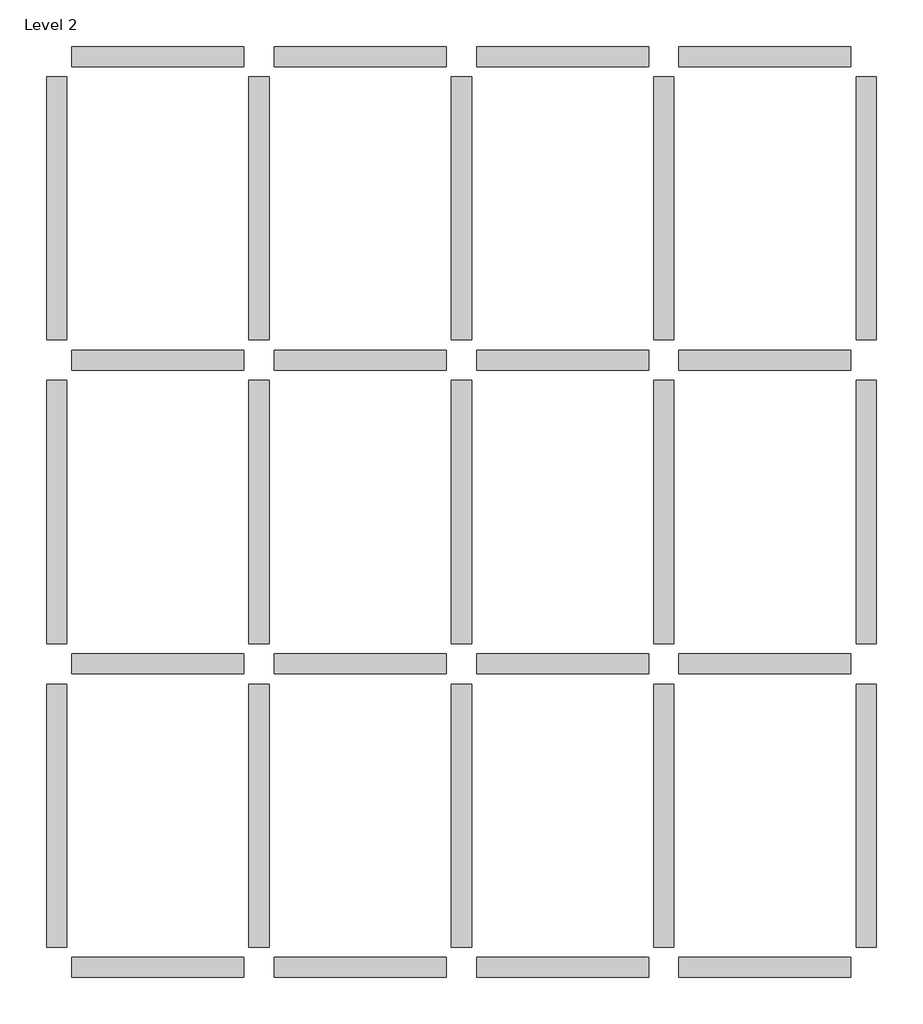
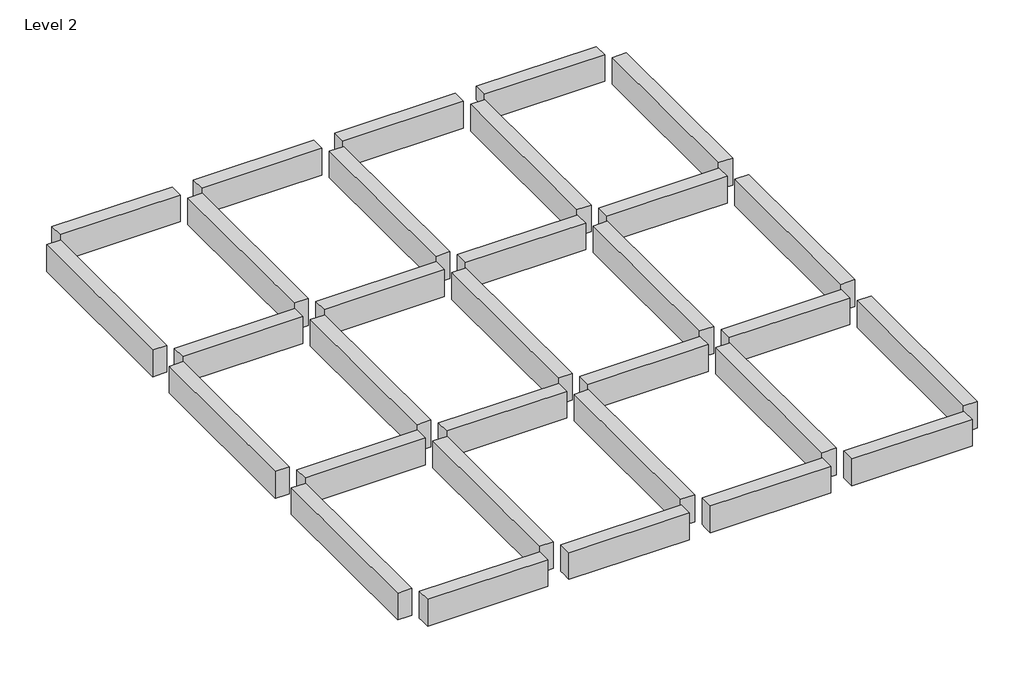
# One storey: 31 beams.
"""IFC4 building model written with IfcOpenShell, lengths in millimetres."""

from ifc_helpers import new_model, si_unit, frame, origin, place, context, project, spatial, polyline, outline, extrude, faceted_brep, element, save

model = new_model("IFC4")

# Units and contexts
model_context = context("Model", 3, world=origin())
ifc_project = project(units=[si_unit("LENGTHUNIT", "METRE", prefix="MILLI")], contexts=[model_context])

# Site, building, storey
site = spatial("IfcSite", under=ifc_project)
building = spatial("IfcBuilding", under=site)
storey = spatial("IfcBuildingStorey", under=building, Name="Level 2", Elevation=3048.0)

# Beams
placement = place(None, origin())
element("IfcBeam", 1, ObjectType="Concrete-Rectangular Beam : 12 x 24", at=placement, inside=storey, context=model_context, shape_type="Brep", body=[
    faceted_brep([(-21467.3183349, 4163.0075069, 3048.0), (-21772.1183349, 4163.0075069, 3048.0), (-21772.1183349, 200.6075069, 3048.0), (-21467.3183349, 200.6075069, 3048.0), (-21467.3183349, 4163.0075069, 2438.4), (-21467.3183349, 200.6075069, 2438.4), (-21772.1183349, 4163.0075069, 2438.4), (-21568.9183349, 4163.0075069, 2438.4), (-21568.9183349, 200.6075069, 2438.4), (-21772.1183349, 200.6075069, 2438.4)], [[[0, 1, 2, 3]], [[4, 0, 3, 5]], [[6, 7, 4, 5, 8, 9]], [[1, 6, 9, 2]], [[1, 0, 4, 7, 6]], [[3, 2, 9, 8, 5]]]),
])
element("IfcBeam", 2, ObjectType="Concrete-Rectangular Beam : 12 x 24", at=placement, inside=storey, context=model_context, shape_type="Brep", body=[
    faceted_brep([(-21467.3183349, 8735.0075069, 3048.0), (-21772.1183349, 8735.0075069, 3048.0), (-21772.1183349, 4772.6075069, 3048.0), (-21467.3183349, 4772.6075069, 3048.0), (-21467.3183349, 8735.0075069, 2438.4), (-21467.3183349, 4772.6075069, 2438.4), (-21772.1183349, 8735.0075069, 2438.4), (-21568.9183349, 8735.0075069, 2438.4), (-21568.9183349, 4772.6075069, 2438.4), (-21772.1183349, 4772.6075069, 2438.4)], [[[0, 1, 2, 3]], [[4, 0, 3, 5]], [[6, 7, 4, 5, 8, 9]], [[1, 6, 9, 2]], [[1, 0, 4, 7, 6]], [[3, 2, 9, 8, 5]]]),
])
element("IfcBeam", 3, ObjectType="Concrete-Rectangular Beam : 12 x 24", at=placement, inside=storey, context=model_context, shape_type="Brep", body=[
    faceted_brep([(-21467.3183349, 13307.0075069, 3048.0), (-21772.1183349, 13307.0075069, 3048.0), (-21772.1183349, 9344.6075069, 3048.0), (-21467.3183349, 9344.6075069, 3048.0), (-21467.3183349, 13307.0075069, 2438.4), (-21467.3183349, 9344.6075069, 2438.4), (-21772.1183349, 13307.0075069, 2438.4), (-21568.9183349, 13307.0075069, 2438.4), (-21568.9183349, 9344.6075069, 2438.4), (-21772.1183349, 9344.6075069, 2438.4)], [[[0, 1, 2, 3]], [[4, 0, 3, 5]], [[6, 7, 4, 5, 8, 9]], [[1, 6, 9, 2]], [[1, 0, 4, 7, 6]], [[3, 2, 9, 8, 5]]]),
])
element("IfcBeam", 4, ObjectType="Concrete-Rectangular Beam : 12 x 24", at=placement, inside=storey, context=model_context, shape_type="SweptSolid", body=[
    extrude(outline(polyline([(-18724.1183349, 4163.0075069), (-18419.3183349, 4163.0075069), (-18419.3183349, 200.6075069), (-18724.1183349, 200.6075069), (-18724.1183349, 4163.0075069)])), frame((0.0, 0.0, 2438.4), z_axis=(0.0, 0.0, 1.0), x_axis=(1.0, 0.0, 0.0)), (0.0, 0.0, 1.0), 609.6),
])
element("IfcBeam", 5, ObjectType="Concrete-Rectangular Beam : 12 x 24", at=placement, inside=storey, context=model_context, shape_type="SweptSolid", body=[
    extrude(outline(polyline([(-18724.1183349, 8735.0075069), (-18419.3183349, 8735.0075069), (-18419.3183349, 4772.6075069), (-18724.1183349, 4772.6075069), (-18724.1183349, 8735.0075069)])), frame((0.0, 0.0, 2438.4), z_axis=(0.0, 0.0, 1.0), x_axis=(1.0, 0.0, 0.0)), (0.0, 0.0, 1.0), 609.6),
])
element("IfcBeam", 6, ObjectType="Concrete-Rectangular Beam : 12 x 24", at=placement, inside=storey, context=model_context, shape_type="SweptSolid", body=[
    extrude(outline(polyline([(-18724.1183349, 13307.0075069), (-18419.3183349, 13307.0075069), (-18419.3183349, 9344.6075069), (-18724.1183349, 9344.6075069), (-18724.1183349, 13307.0075069)])), frame((0.0, 0.0, 2438.4), z_axis=(0.0, 0.0, 1.0), x_axis=(1.0, 0.0, 0.0)), (0.0, 0.0, 1.0), 609.6),
])
element("IfcBeam", 7, ObjectType="Concrete-Rectangular Beam : 12 x 24", at=placement, inside=storey, context=model_context, shape_type="SweptSolid", body=[
    extrude(outline(polyline([(-15676.1183349, 4163.0075069), (-15371.3183349, 4163.0075069), (-15371.3183349, 200.6075069), (-15676.1183349, 200.6075069), (-15676.1183349, 4163.0075069)])), frame((0.0, 0.0, 2438.4), z_axis=(0.0, 0.0, 1.0), x_axis=(1.0, 0.0, 0.0)), (0.0, 0.0, 1.0), 609.6),
])
element("IfcBeam", 8, ObjectType="Concrete-Rectangular Beam : 12 x 24", at=placement, inside=storey, context=model_context, shape_type="SweptSolid", body=[
    extrude(outline(polyline([(-15676.1183349, 8735.0075069), (-15371.3183349, 8735.0075069), (-15371.3183349, 4772.6075069), (-15676.1183349, 4772.6075069), (-15676.1183349, 8735.0075069)])), frame((0.0, 0.0, 2438.4), z_axis=(0.0, 0.0, 1.0), x_axis=(1.0, 0.0, 0.0)), (0.0, 0.0, 1.0), 609.6),
])
element("IfcBeam", 9, ObjectType="Concrete-Rectangular Beam : 12 x 24", at=placement, inside=storey, context=model_context, shape_type="SweptSolid", body=[
    extrude(outline(polyline([(-15676.1183349, 13307.0075069), (-15371.3183349, 13307.0075069), (-15371.3183349, 9344.6075069), (-15676.1183349, 9344.6075069), (-15676.1183349, 13307.0075069)])), frame((0.0, 0.0, 2438.4), z_axis=(0.0, 0.0, 1.0), x_axis=(1.0, 0.0, 0.0)), (0.0, 0.0, 1.0), 609.6),
])
element("IfcBeam", 10, ObjectType="Concrete-Rectangular Beam : 12 x 24", at=placement, inside=storey, context=model_context, shape_type="SweptSolid", body=[
    extrude(outline(polyline([(-12628.1183349, 4163.0075069), (-12323.3183349, 4163.0075069), (-12323.3183349, 200.6075069), (-12628.1183349, 200.6075069), (-12628.1183349, 4163.0075069)])), frame((0.0, 0.0, 2438.4), z_axis=(0.0, 0.0, 1.0), x_axis=(1.0, 0.0, 0.0)), (0.0, 0.0, 1.0), 609.6),
])
element("IfcBeam", 11, ObjectType="Concrete-Rectangular Beam : 12 x 24", at=placement, inside=storey, context=model_context, shape_type="SweptSolid", body=[
    extrude(outline(polyline([(-12628.1183349, 8735.0075069), (-12323.3183349, 8735.0075069), (-12323.3183349, 4772.6075069), (-12628.1183349, 4772.6075069), (-12628.1183349, 8735.0075069)])), frame((0.0, 0.0, 2438.4), z_axis=(0.0, 0.0, 1.0), x_axis=(1.0, 0.0, 0.0)), (0.0, 0.0, 1.0), 609.6),
])
element("IfcBeam", 12, ObjectType="Concrete-Rectangular Beam : 12 x 24", at=placement, inside=storey, context=model_context, shape_type="SweptSolid", body=[
    extrude(outline(polyline([(-12628.1183349, 13307.0075069), (-12323.3183349, 13307.0075069), (-12323.3183349, 9344.6075069), (-12628.1183349, 9344.6075069), (-12628.1183349, 13307.0075069)])), frame((0.0, 0.0, 2438.4), z_axis=(0.0, 0.0, 1.0), x_axis=(1.0, 0.0, 0.0)), (0.0, 0.0, 1.0), 609.6),
])
element("IfcBeam", 13, ObjectType="Concrete-Rectangular Beam : 12 x 24", at=placement, inside=storey, context=model_context, shape_type="Brep", body=[
    faceted_brep([(-9275.3183349, 4163.0075069, 3048.0), (-9580.1183349, 4163.0075069, 3048.0), (-9580.1183349, 200.6075069, 3048.0), (-9275.3183349, 200.6075069, 3048.0), (-9275.3183349, 4163.0075069, 2438.4), (-9275.3183349, 200.6075069, 2438.4), (-9580.1183349, 4163.0075069, 2438.4), (-9478.5183349, 4163.0075069, 2438.4), (-9478.5183349, 200.6075069, 2438.4), (-9580.1183349, 200.6075069, 2438.4)], [[[0, 1, 2, 3]], [[4, 0, 3, 5]], [[6, 7, 4, 5, 8, 9]], [[1, 6, 9, 2]], [[1, 0, 4, 7, 6]], [[3, 2, 9, 8, 5]]]),
])
element("IfcBeam", 14, ObjectType="Concrete-Rectangular Beam : 12 x 24", at=placement, inside=storey, context=model_context, shape_type="Brep", body=[
    faceted_brep([(-9275.3183349, 8735.0075069, 3048.0), (-9580.1183349, 8735.0075069, 3048.0), (-9580.1183349, 4772.6075069, 3048.0), (-9275.3183349, 4772.6075069, 3048.0), (-9275.3183349, 8735.0075069, 2438.4), (-9275.3183349, 4772.6075069, 2438.4), (-9580.1183349, 8735.0075069, 2438.4), (-9478.5183349, 8735.0075069, 2438.4), (-9478.5183349, 4772.6075069, 2438.4), (-9580.1183349, 4772.6075069, 2438.4)], [[[0, 1, 2, 3]], [[4, 0, 3, 5]], [[6, 7, 4, 5, 8, 9]], [[1, 6, 9, 2]], [[1, 0, 4, 7, 6]], [[3, 2, 9, 8, 5]]]),
])
element("IfcBeam", 15, ObjectType="Concrete-Rectangular Beam : 12 x 24", at=placement, inside=storey, context=model_context, shape_type="Brep", body=[
    faceted_brep([(-9275.3183349, 13307.0075069, 3048.0), (-9580.1183349, 13307.0075069, 3048.0), (-9580.1183349, 9344.6075069, 3048.0), (-9275.3183349, 9344.6075069, 3048.0), (-9275.3183349, 13307.0075069, 2438.4), (-9275.3183349, 9344.6075069, 2438.4), (-9580.1183349, 13307.0075069, 2438.4), (-9478.5183349, 13307.0075069, 2438.4), (-9478.5183349, 9344.6075069, 2438.4), (-9580.1183349, 9344.6075069, 2438.4)], [[[0, 1, 2, 3]], [[4, 0, 3, 5]], [[6, 7, 4, 5, 8, 9]], [[1, 6, 9, 2]], [[1, 0, 4, 7, 6]], [[3, 2, 9, 8, 5]]]),
])
element("IfcBeam", 16, ObjectType="Concrete-Rectangular Beam : 12 x 24", at=placement, inside=storey, context=model_context, shape_type="Brep", body=[
    faceted_brep([(-21391.1183349, 13764.2075069, 3048.0), (-21391.1183349, 13459.4075069, 3048.0), (-18800.3183349, 13459.4075069, 3048.0), (-18800.3183349, 13764.2075069, 3048.0), (-21391.1183349, 13459.4075069, 2438.4), (-18800.3183349, 13459.4075069, 2438.4), (-21391.1183349, 13561.0075069, 2438.4), (-21391.1183349, 13764.2075069, 2438.4), (-18800.3183349, 13764.2075069, 2438.4), (-18800.3183349, 13561.0075069, 2438.4)], [[[0, 1, 2, 3]], [[1, 4, 5, 2]], [[4, 6, 7, 8, 9, 5]], [[7, 0, 3, 8]], [[1, 0, 7, 6, 4]], [[3, 2, 5, 9, 8]]]),
])
element("IfcBeam", 17, ObjectType="Concrete-Rectangular Beam : 12 x 24", at=placement, inside=storey, context=model_context, shape_type="Brep", body=[
    faceted_brep([(-18343.1183349, 13764.2075069, 3048.0), (-18343.1183349, 13459.4075069, 3048.0), (-15752.3183349, 13459.4075069, 3048.0), (-15752.3183349, 13764.2075069, 3048.0), (-18343.1183349, 13459.4075069, 2438.4), (-15752.3183349, 13459.4075069, 2438.4), (-18343.1183349, 13561.0075069, 2438.4), (-18343.1183349, 13764.2075069, 2438.4), (-15752.3183349, 13764.2075069, 2438.4), (-15752.3183349, 13561.0075069, 2438.4)], [[[0, 1, 2, 3]], [[1, 4, 5, 2]], [[4, 6, 7, 8, 9, 5]], [[7, 0, 3, 8]], [[1, 0, 7, 6, 4]], [[3, 2, 5, 9, 8]]]),
])
element("IfcBeam", 18, ObjectType="Concrete-Rectangular Beam : 12 x 24", at=placement, inside=storey, context=model_context, shape_type="Brep", body=[
    faceted_brep([(-15295.1183349, 13764.2075069, 3048.0), (-15295.1183349, 13459.4075069, 3048.0), (-12704.3183349, 13459.4075069, 3048.0), (-12704.3183349, 13764.2075069, 3048.0), (-15295.1183349, 13459.4075069, 2438.4), (-12704.3183349, 13459.4075069, 2438.4), (-15295.1183349, 13561.0075069, 2438.4), (-15295.1183349, 13764.2075069, 2438.4), (-12704.3183349, 13764.2075069, 2438.4), (-12704.3183349, 13561.0075069, 2438.4)], [[[0, 1, 2, 3]], [[1, 4, 5, 2]], [[4, 6, 7, 8, 9, 5]], [[7, 0, 3, 8]], [[1, 0, 7, 6, 4]], [[3, 2, 5, 9, 8]]]),
])
element("IfcBeam", 19, ObjectType="Concrete-Rectangular Beam : 12 x 24", at=placement, inside=storey, context=model_context, shape_type="SweptSolid", body=[
    extrude(outline(polyline([(13459.4075069, 3048.0), (13764.2075069, 3048.0), (13764.2075069, 2743.2), (13561.0075069, 2743.2), (13561.0075069, 2438.4), (13459.4075069, 2438.4), (13459.4075069, 3048.0)])), frame((-12247.1183349, 0.0, 0.0), z_axis=(1.0, 0.0, 0.0), x_axis=(0.0, 1.0, 0.0)), (0.0, 0.0, 1.0), 2590.8),
])
element("IfcBeam", 20, ObjectType="Concrete-Rectangular Beam : 12 x 24", at=placement, inside=storey, context=model_context, shape_type="SweptSolid", body=[
    extrude(outline(polyline([(-21391.1183349, 8887.4075069), (-21391.1183349, 9192.2075069), (-18800.3183349, 9192.2075069), (-18800.3183349, 8887.4075069), (-21391.1183349, 8887.4075069)])), frame((0.0, 0.0, 2438.4), z_axis=(0.0, 0.0, 1.0), x_axis=(1.0, 0.0, 0.0)), (0.0, 0.0, 1.0), 609.6),
])
element("IfcBeam", 21, ObjectType="Concrete-Rectangular Beam : 12 x 24", at=placement, inside=storey, context=model_context, shape_type="SweptSolid", body=[
    extrude(outline(polyline([(-18343.1183349, 8887.4075069), (-18343.1183349, 9192.2075069), (-15752.3183349, 9192.2075069), (-15752.3183349, 8887.4075069), (-18343.1183349, 8887.4075069)])), frame((0.0, 0.0, 2438.4), z_axis=(0.0, 0.0, 1.0), x_axis=(1.0, 0.0, 0.0)), (0.0, 0.0, 1.0), 609.6),
])
element("IfcBeam", 22, ObjectType="Concrete-Rectangular Beam : 12 x 24", at=placement, inside=storey, context=model_context, shape_type="SweptSolid", body=[
    extrude(outline(polyline([(-15295.1183349, 8887.4075069), (-15295.1183349, 9192.2075069), (-12704.3183349, 9192.2075069), (-12704.3183349, 8887.4075069), (-15295.1183349, 8887.4075069)])), frame((0.0, 0.0, 2438.4), z_axis=(0.0, 0.0, 1.0), x_axis=(1.0, 0.0, 0.0)), (0.0, 0.0, 1.0), 609.6),
])
element("IfcBeam", 23, ObjectType="Concrete-Rectangular Beam : 12 x 24", at=placement, inside=storey, context=model_context, shape_type="SweptSolid", body=[
    extrude(outline(polyline([(-12247.1183349, 8887.4075069), (-12247.1183349, 9192.2075069), (-9656.3183349, 9192.2075069), (-9656.3183349, 8887.4075069), (-12247.1183349, 8887.4075069)])), frame((0.0, 0.0, 2438.4), z_axis=(0.0, 0.0, 1.0), x_axis=(1.0, 0.0, 0.0)), (0.0, 0.0, 1.0), 609.6),
])
element("IfcBeam", 24, ObjectType="Concrete-Rectangular Beam : 12 x 24", at=placement, inside=storey, context=model_context, shape_type="SweptSolid", body=[
    extrude(outline(polyline([(-21391.1183349, 4315.4075069), (-21391.1183349, 4620.2075069), (-18800.3183349, 4620.2075069), (-18800.3183349, 4315.4075069), (-21391.1183349, 4315.4075069)])), frame((0.0, 0.0, 2438.4), z_axis=(0.0, 0.0, 1.0), x_axis=(1.0, 0.0, 0.0)), (0.0, 0.0, 1.0), 609.6),
])
element("IfcBeam", 25, ObjectType="Concrete-Rectangular Beam : 12 x 24", at=placement, inside=storey, context=model_context, shape_type="SweptSolid", body=[
    extrude(outline(polyline([(-18343.1183349, 4315.4075069), (-18343.1183349, 4620.2075069), (-15752.3183349, 4620.2075069), (-15752.3183349, 4315.4075069), (-18343.1183349, 4315.4075069)])), frame((0.0, 0.0, 2438.4), z_axis=(0.0, 0.0, 1.0), x_axis=(1.0, 0.0, 0.0)), (0.0, 0.0, 1.0), 609.6),
])
element("IfcBeam", 26, ObjectType="Concrete-Rectangular Beam : 12 x 24", at=placement, inside=storey, context=model_context, shape_type="SweptSolid", body=[
    extrude(outline(polyline([(-15295.1183349, 4315.4075069), (-15295.1183349, 4620.2075069), (-12704.3183349, 4620.2075069), (-12704.3183349, 4315.4075069), (-15295.1183349, 4315.4075069)])), frame((0.0, 0.0, 2438.4), z_axis=(0.0, 0.0, 1.0), x_axis=(1.0, 0.0, 0.0)), (0.0, 0.0, 1.0), 609.6),
])
element("IfcBeam", 27, ObjectType="Concrete-Rectangular Beam : 12 x 24", at=placement, inside=storey, context=model_context, shape_type="SweptSolid", body=[
    extrude(outline(polyline([(-12247.1183349, 4315.4075069), (-12247.1183349, 4620.2075069), (-9656.3183349, 4620.2075069), (-9656.3183349, 4315.4075069), (-12247.1183349, 4315.4075069)])), frame((0.0, 0.0, 2438.4), z_axis=(0.0, 0.0, 1.0), x_axis=(1.0, 0.0, 0.0)), (0.0, 0.0, 1.0), 609.6),
])
element("IfcBeam", 28, ObjectType="Concrete-Rectangular Beam : 12 x 24", at=placement, inside=storey, context=model_context, shape_type="Brep", body=[
    faceted_brep([(-21391.1183349, 48.2075069, 3048.0), (-21391.1183349, -256.5924931, 3048.0), (-18800.3183349, -256.5924931, 3048.0), (-18800.3183349, 48.2075069, 3048.0), (-21391.1183349, -256.5924931, 2438.4), (-18800.3183349, -256.5924931, 2438.4), (-21391.1183349, -53.3924931, 2438.4), (-21391.1183349, 48.2075069, 2438.4), (-18800.3183349, 48.2075069, 2438.4), (-18800.3183349, -53.3924931, 2438.4)], [[[0, 1, 2, 3]], [[1, 4, 5, 2]], [[4, 6, 7, 8, 9, 5]], [[7, 0, 3, 8]], [[1, 0, 7, 6, 4]], [[3, 2, 5, 9, 8]]]),
])
element("IfcBeam", 29, ObjectType="Concrete-Rectangular Beam : 12 x 24", at=placement, inside=storey, context=model_context, shape_type="Brep", body=[
    faceted_brep([(-18343.1183349, 48.2075069, 3048.0), (-18343.1183349, -256.5924931, 3048.0), (-15752.3183349, -256.5924931, 3048.0), (-15752.3183349, 48.2075069, 3048.0), (-18343.1183349, -256.5924931, 2438.4), (-15752.3183349, -256.5924931, 2438.4), (-18343.1183349, -53.3924931, 2438.4), (-18343.1183349, 48.2075069, 2438.4), (-15752.3183349, 48.2075069, 2438.4), (-15752.3183349, -53.3924931, 2438.4)], [[[0, 1, 2, 3]], [[1, 4, 5, 2]], [[4, 6, 7, 8, 9, 5]], [[7, 0, 3, 8]], [[1, 0, 7, 6, 4]], [[3, 2, 5, 9, 8]]]),
])
element("IfcBeam", 30, ObjectType="Concrete-Rectangular Beam : 12 x 24", at=placement, inside=storey, context=model_context, shape_type="Brep", body=[
    faceted_brep([(-15295.1183349, 48.2075069, 3048.0), (-15295.1183349, -256.5924931, 3048.0), (-12704.3183349, -256.5924931, 3048.0), (-12704.3183349, 48.2075069, 3048.0), (-15295.1183349, -256.5924931, 2438.4), (-12704.3183349, -256.5924931, 2438.4), (-15295.1183349, -53.3924931, 2438.4), (-15295.1183349, 48.2075069, 2438.4), (-12704.3183349, 48.2075069, 2438.4), (-12704.3183349, -53.3924931, 2438.4)], [[[0, 1, 2, 3]], [[1, 4, 5, 2]], [[4, 6, 7, 8, 9, 5]], [[7, 0, 3, 8]], [[1, 0, 7, 6, 4]], [[3, 2, 5, 9, 8]]]),
])
element("IfcBeam", 31, ObjectType="Concrete-Rectangular Beam : 12 x 24", at=placement, inside=storey, context=model_context, shape_type="Brep", body=[
    faceted_brep([(-12247.1183349, 48.2075069, 3048.0), (-12247.1183349, -256.5924931, 3048.0), (-9656.3183349, -256.5924931, 3048.0), (-9656.3183349, 48.2075069, 3048.0), (-12247.1183349, -256.5924931, 2438.4), (-9656.3183349, -256.5924931, 2438.4), (-12247.1183349, -53.3924931, 2438.4), (-12247.1183349, 48.2075069, 2438.4), (-9656.3183349, 48.2075069, 2438.4), (-9656.3183349, -53.3924931, 2438.4)], [[[0, 1, 2, 3]], [[1, 4, 5, 2]], [[4, 6, 7, 8, 9, 5]], [[7, 0, 3, 8]], [[1, 0, 7, 6, 4]], [[3, 2, 5, 9, 8]]]),
])

save(model, "model.ifc")

# Revit data of these elements
# Type "Concrete-Rectangular Beam : 12 x 24"
#   Assembly Code = "B10"
#   Length [instance default] = 5' - 0"
#   b = 1' - 0"
#   h = 2' - 0"
#   Structural Material [instance default] = Concrete, Cast-in-Place gray
# Elements 1, 2, 3, 4, 5, 6, 7, 8, 9, 10, 11, 12, 13, 14, 15, 16, 17, 18, 19, 20, 21, 22, 23, 24, 25, 26, 27, 28, 29, 30, 31 (IfcBeam, "Concrete-Rectangular Beam : 12 x 24")
#   Structural Material = Concrete, Cast-in-Place gray
#   Phase Created = New Construction
#   Materials on its faces: "Concrete, Cast-in-Place gray"
# Materials
#   "Concrete, Cast-in-Place gray": class "Concrete", colour RGB 192 192 192, transparency 0, Description = "Cast-in-place concrete", Cost = 0
